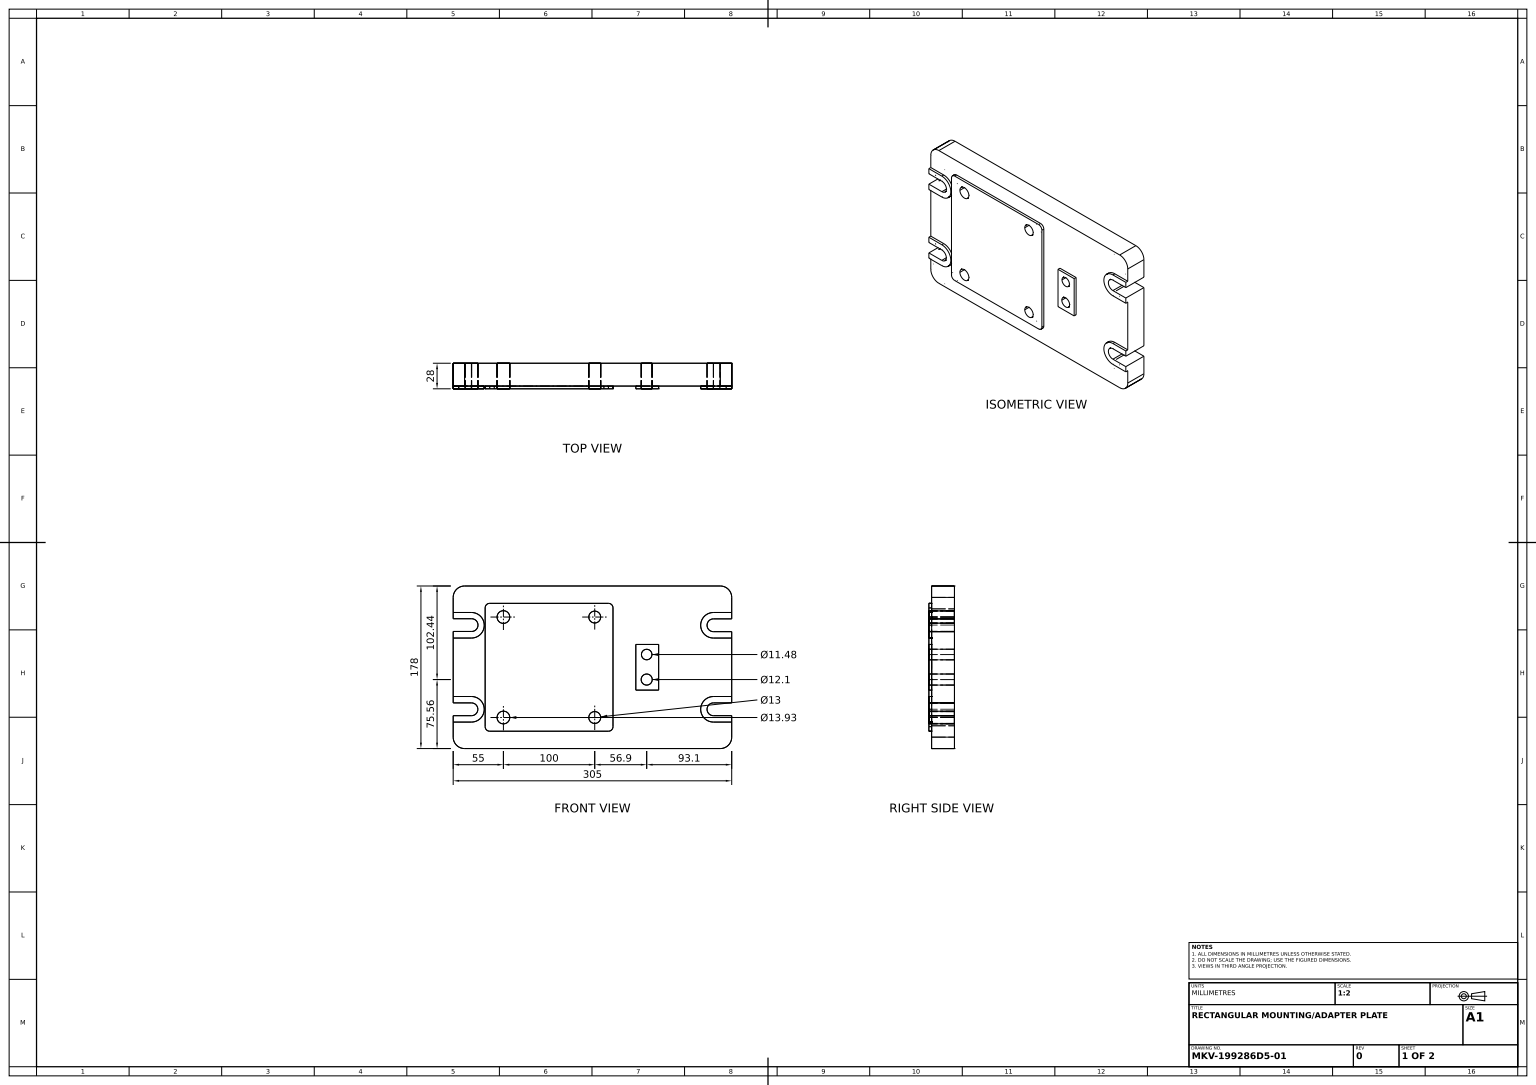
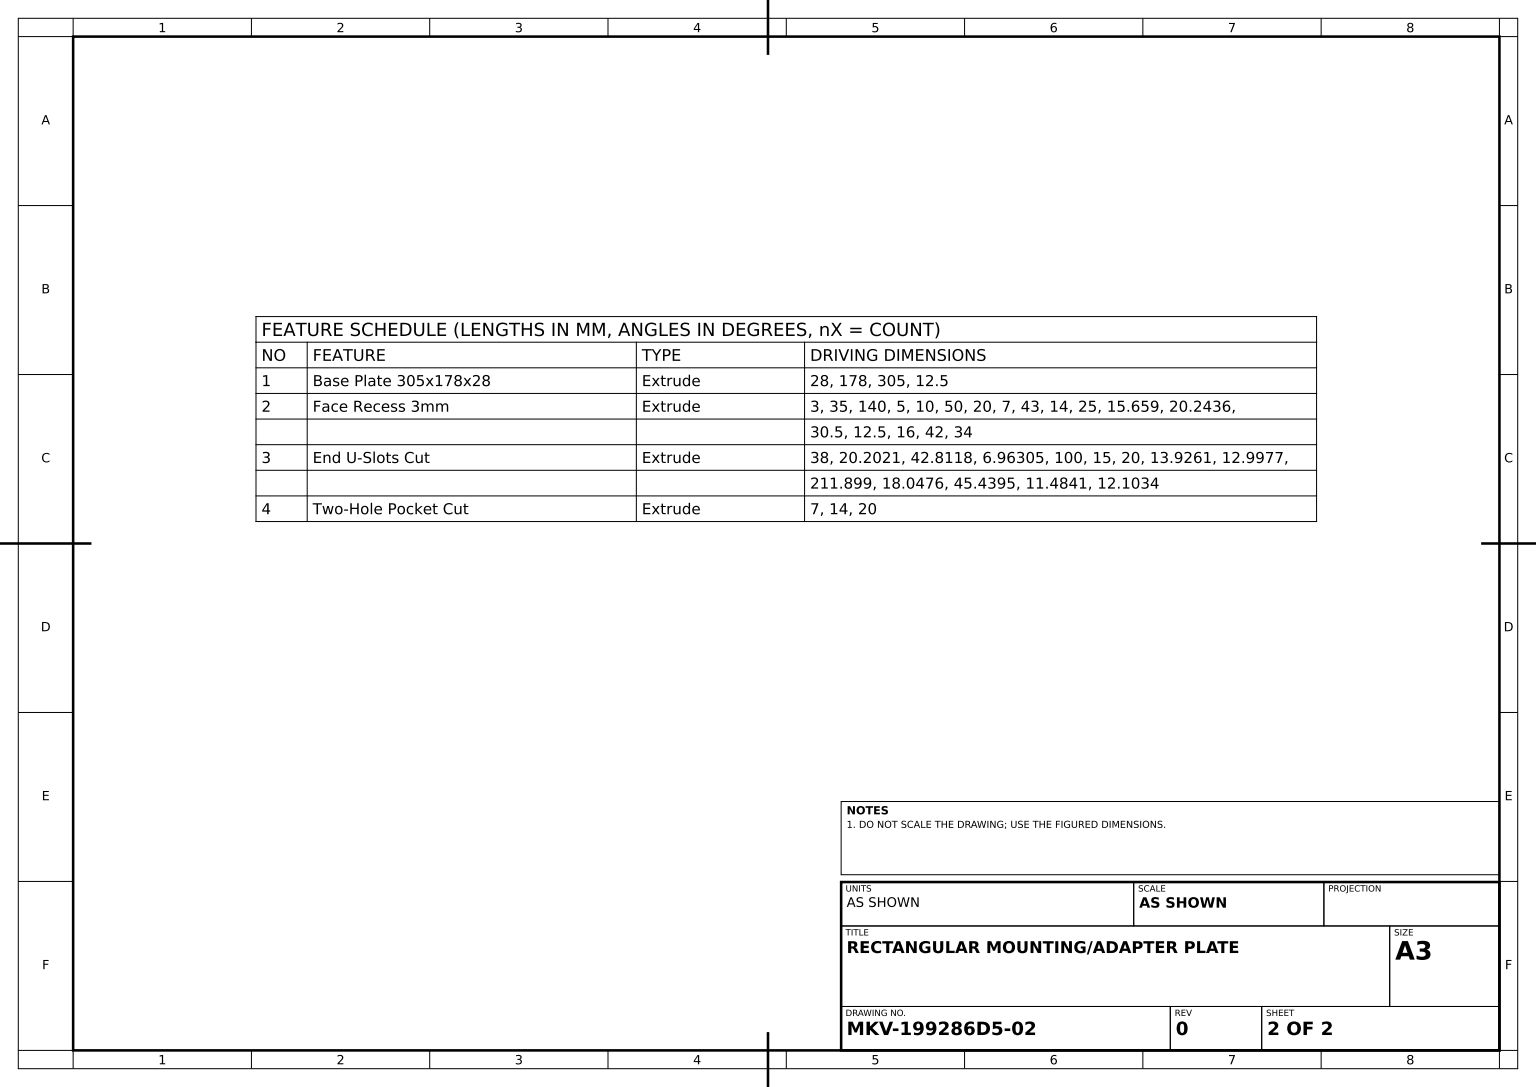
SolidWorks part; units mm, degrees
material "Plain Carbon Steel"
ref_plane "Front Plane" through (0, 0, 0) normal (0, 0, 1) x (1, 0, 0)
ref_plane "Top Plane" through (0, 0, 0) normal (0, 1, 0) x (1, 0, 0)
ref_plane "Right Plane" through (0, 0, 0) normal (1, 0, 0) x (0, 0, -1)
sketch "Base Plate Profile" plane through (0, 0, 0) normal (0, 0, 1) x (1, 0, 0)
  line L0 (0, 139.0067) -> (0, -168.1773) construction
  line L1 (-293.4916, 0) -> (285.7525, 0) construction
  line L3 (-140, 89) -> (140, 89)
  line L4 (-152.5, 76.5) -> (-152.5, -76.5)
  line L5 (-140, -89) -> (140, -89)
  line L6 (152.5, 76.5) -> (152.5, -76.5)
  line L7 (-152.5, 89) -> (152.5, -89) construction
  line L8 (-152.5, -89) -> (152.5, 89) construction
  arc A0 (-152.5, -76.5) -> (-140, -89) centre (-140, -76.5) ccw
  arc A1 (140, -89) -> (152.5, -76.5) centre (140, -76.5) ccw
  arc A2 (140, 89) -> (152.5, 76.5) centre (140, 76.5) cw
  arc A3 (-140, 89) -> (-152.5, 76.5) centre (-140, 76.5) ccw
  point P5 (0, 0)
  dimension "D3" = 12.5
  dimension "D1" = 178
  dimension "D2" = 305
extrude "Base Plate 305x178x28" add sketch "Base Plate Profile" along normal mid plane 28
sketch "Face Recess Profile" plane through (0, 0, 14) normal (0, 0, 1) x (1, 0, 0)
  line L0 (-140, -89) -> (140, -89) construction
  line L1 (-112.5, 70) -> (17.5, 70)
  line L2 (-117.5, 65) -> (-117.5, -65)
  line L3 (-112.5, -70) -> (17.5, -70)
  line L4 (22.5, 65) -> (22.5, -65)
  line L5 (-117.5, 70) -> (22.5, -70) construction
  line L6 (-117.5, -70) -> (22.5, 70) construction
  line L7 (-152.5, 76.5) -> (-152.5, -76.5) construction
  line L8 (140, 89) -> (-140, 89) construction
  line L9 (-140, -89) -> (140, -89)
  line L10 (-152.5, 76.5) -> (-152.5, -76.5)
  line L11 (140, 89) -> (-140, 89)
  line L12 (-47.5, 106.7781) -> (-47.5, -39) construction
  line L13 (-140, 0) -> (17.5, 0) construction
  line L14 (-152.5, 53) -> (-132.5, 53)
  line L15 (-152.5, 39) -> (-132.5, 39)
  line L16 (-152.5, 60) -> (-132.5, 60)
  line L17 (-152.5, 32) -> (-132.5, 32)
  line L18 (-152.5, -39) -> (-132.5, -39)
  line L19 (-152.5, -53) -> (-132.5, -53)
  line L20 (-152.5, -32) -> (-132.5, -32)
  line L21 (-152.5, -60) -> (-132.5, -60)
  line L22 (17.5, 0) -> (102.5, 0) construction
  line L23 (47.5, 25) -> (72.5, 25)
  line L24 (47.5, 25) -> (47.5, -25)
  line L25 (47.5, -25) -> (72.5, -25)
  line L26 (72.5, 25) -> (72.5, -25)
  line L27 (47.5, 25) -> (72.5, -25) construction
  line L28 (47.5, -25) -> (72.5, 25) construction
  line L30 (152.5, -60) -> (132.5, -60)
  line L31 (152.5, -53) -> (132.5, -53)
  line L32 (152.5, -39) -> (132.5, -39)
  line L33 (152.5, -32) -> (132.5, -32)
  line L34 (152.5, 32) -> (132.5, 32)
  line L35 (152.5, 39) -> (132.5, 39)
  line L36 (152.5, 53) -> (132.5, 53)
  line L37 (152.7436, 60) -> (132.5, 60)
  line L38 (152.5, -76.5) -> (152.5, 76.5) construction
  arc A0 (152.5, 76.5) -> (140, 89) centre (140, 76.5) ccw construction
  arc A1 (140, -89) -> (152.5, -76.5) centre (140, -76.5) ccw construction
  arc A2 (-152.5, -76.5) -> (-140, -89) centre (-140, -76.5) ccw construction
  arc A3 (-140, 89) -> (-152.5, 76.5) centre (-140, 76.5) ccw construction
  arc A4 (152.5, 76.5) -> (140, 89) centre (140, 76.5) ccw
  arc A5 (140, -89) -> (152.5, -76.5) centre (140, -76.5) ccw
  arc A6 (-152.5, -76.5) -> (-140, -89) centre (-140, -76.5) ccw
  arc A7 (-140, 89) -> (-152.5, 76.5) centre (-140, 76.5) ccw
  arc A8 (17.5, -70) -> (22.5, -65) centre (17.5, -65) ccw
  arc A9 (-117.5, -65) -> (-112.5, -70) centre (-112.5, -65) ccw
  arc A10 (17.5, 70) -> (22.5, 65) centre (17.5, 65) cw
  arc A11 (-112.5, 70) -> (-117.5, 65) centre (-112.5, 65) ccw
  circle A12 centre (-97.5, 50) radius 5
  circle A13 centre (2.5, 50) radius 5
  circle A14 centre (2.5, -50) radius 5
  circle A15 centre (-97.5, -50) radius 5
  arc A16 (-132.5, 53) -> (-132.5, 39) centre (-132.5, 46) cw
  arc A17 (-132.5, 60) -> (-132.5, 32) centre (-132.5, 46) cw
  arc A18 (-132.5, -39) -> (-132.5, -53) centre (-132.5, -46) cw
  arc A19 (-132.5, -32) -> (-132.5, -60) centre (-132.5, -46) cw
  circle A20 centre (60, 15.659) radius 7.0029
  circle A21 centre (60, -17) radius 8
  arc A22 (132.5, -39) -> (132.5, -53) centre (132.5, -46) ccw
  arc A23 (132.5, -32) -> (132.5, -60) centre (132.5, -46) ccw
  arc A24 (132.5, 53) -> (132.5, 39) centre (132.5, 46) ccw
  arc A25 (132.5, 60) -> (132.5, 32) centre (132.5, 46) ccw
  point P0 (-47.5, 0)
  point P62 (60, 0)
  point P94 (118.5, 46)
  arc M32 (-152.5, -76.5) -> (-140, -89) centre (-140, -76.5) ccw
  line M33 (-140, -89) -> (140, -89)
  arc M34 (140, -89) -> (152.5, -76.5) centre (140, -76.5) ccw
  line M35 (152.5, -76.5) -> (152.5, 76.5)
  arc M36 (152.5, 76.5) -> (140, 89) centre (140, 76.5) ccw
  line M37 (140, 89) -> (-140, 89)
  arc M38 (-140, 89) -> (-152.5, 76.5) centre (-140, 76.5) ccw
  line M39 (-152.5, 76.5) -> (-152.5, -76.5)
  dimension "D4" = 5
  dimension "D5" = 10
  dimension "D10" = 7
  dimension "D20" = 14
  dimension "D28" = 7
  dimension "D29" = 14
  dimension "D32" = 12.5
  dimension "D33" = 16
  dimension "D36" = 34
  dimension "D1" = 35
  dimension "D2" = 140
  dimension "D3" = 140
  dimension "D6" = 50
  dimension "D7" = 50
  dimension "D8" = 20
  dimension "D9" = 20
  dimension "D11" = 43
  dimension "D12" = 7
  dimension "D13" = 20
  dimension "D14" = 7
  dimension "D15" = 14
  dimension "D16" = 20
  dimension "D17" = 43
  dimension "D18" = 7
  dimension "D19" = 7
  dimension "D21" = 50
  dimension "D22" = 25
  dimension "D23" = 25
  dimension "D24" = 15.659
  dimension "D25" = 20
  dimension "D26" = 20.2436
  dimension "D27" = 30.5
  dimension "D30" = 43
  dimension "D31" = 165.5
  dimension "D34" = 12.5
  dimension "D35" = 42
extrude "Face Recess 3mm" cut sketch "Face Recess Profile" against normal blind 3 contours A25 L37 L16 A17 L17 L10 L20 A19 L21 L30 A23 L33 L34 A11 L1 A10 L4 A8 L3 A9 L2 L23 L26 L25 L24 M35 M36 M37 M38 M39 M32 M33 M34
sketch "End Slots Profile" plane through (0, 0, 14) normal (0, 0, 1) x (1, 0, 0)
  line L0 (-152.5, 53.1513) -> (-132.2979, 53.1513)
  line L1 (-152.5, 60) -> (-152.5, 32) construction
  line L2 (0, 46.1882) -> (0, -44.3314) construction
  line L3 (-132.2979, 39.2252) -> (-152.5, 39.2252)
  line L4 (-132.2979, 0) -> (116.9792, 0) construction
  line L5 (-132.2979, -39.2252) -> (-152.5, -39.2252)
  line L6 (-152.5, -53.1513) -> (-132.2979, -53.1513)
  line L7 (132.2979, 39.2252) -> (152.5, 39.2252)
  line L8 (152.5, -53.1513) -> (132.2979, -53.1513)
  line L9 (132.2979, -39.2252) -> (152.5, -39.2252)
  line L10 (152.5, 53.1513) -> (132.2979, 53.1513)
  line L11 (-112.5, 70) -> (17.5, 70) construction
  line L12 (22.5, 65) -> (22.5, -65) construction
  line L13 (-152.5, 32) -> (-132.5, 32) construction
  arc A0 (-132.2979, 53.1513) -> (-132.2979, 39.2252) centre (-132.2979, 46.1882) cw
  arc A1 (-132.2979, -53.1513) -> (-132.2979, -39.2252) centre (-132.2979, -46.1882) ccw
  arc A2 (132.2979, 53.1513) -> (132.2979, 39.2252) centre (132.2979, 46.1882) ccw
  arc A3 (132.2979, -53.1513) -> (132.2979, -39.2252) centre (132.2979, -46.1882) cw
  circle A4 centre (-97.5, 55) radius 6.963
  circle A5 centre (2.5, 55) radius 6.4988
  circle A8 centre (2.5, -55) radius 6.4988
  circle A9 centre (-97.5, -55) radius 6.963
  circle A10 centre (59.3989, 13.9524) radius 5.742
  circle A11 centre (59.3989, -13.4395) radius 6.0517
  line M12 (-152.5, 60) -> (-152.5, 32)
  dimension "D3" = 6.963
  dimension "D5" = 13.9261
  dimension "D8" = 12.9977
  dimension "D14" = 11.4841
  dimension "D15" = 12.1034
  dimension "D1" = 20.2021
  dimension "D2" = 42.8118
  dimension "D4" = 100
  dimension "D6" = 15
  dimension "D7" = 20
  dimension "D9" = 20
  dimension "D10" = 211.8989
  dimension "D11" = 28
  dimension "D12" = 18.0476
  dimension "D13" = 45.4395
extrude "End U-Slots Cut" cut sketch "End Slots Profile" against normal blind 38 contours A0 L0 L3 M12 | A4 | A5 | A8 | A10 | A9 | A11
sketch "Hole Pocket Profile" plane through (0, 0, 14) normal (0, 0, 1) x (1, 0, 0)
  line L0 (-152.5, -39) -> (-132.5, -39)
  line L1 (-152.5, -32) -> (-152.5, -60) construction
  line L2 (-152.5, -53) -> (-132.5, -53)
  line L3 (-152.5, -32) -> (-132.5, -32) construction
  line L5 (-152.5, -39) -> (-152.5, -53)
  line L6 (0, -15.4) -> (0, 15.4) construction
  line L7 (152.5, -39) -> (152.5, -53)
  line L8 (152.5, -53) -> (132.5, -53)
  line L9 (152.5, -39) -> (132.5, -39)
  line L10 (15.4, 0) -> (-15.4, 0) construction
  line L11 (152.5, 39) -> (132.5, 39)
  line L12 (152.5, 53) -> (132.5, 53)
  line L13 (152.5, 39) -> (152.5, 53)
  arc A0 (-132.5, -39) -> (-132.5, -53) centre (-132.5, -46) cw
  arc A1 (132.5, -39) -> (132.5, -53) centre (132.5, -46) ccw
  arc A2 (132.5, 39) -> (132.5, 53) centre (132.5, 46) cw
  dimension "D3" = 20
  dimension "D1" = 7
  dimension "D2" = 14
extrude "Two-Hole Pocket Cut" cut sketch "Hole Pocket Profile" against normal through all both and the other way through all
